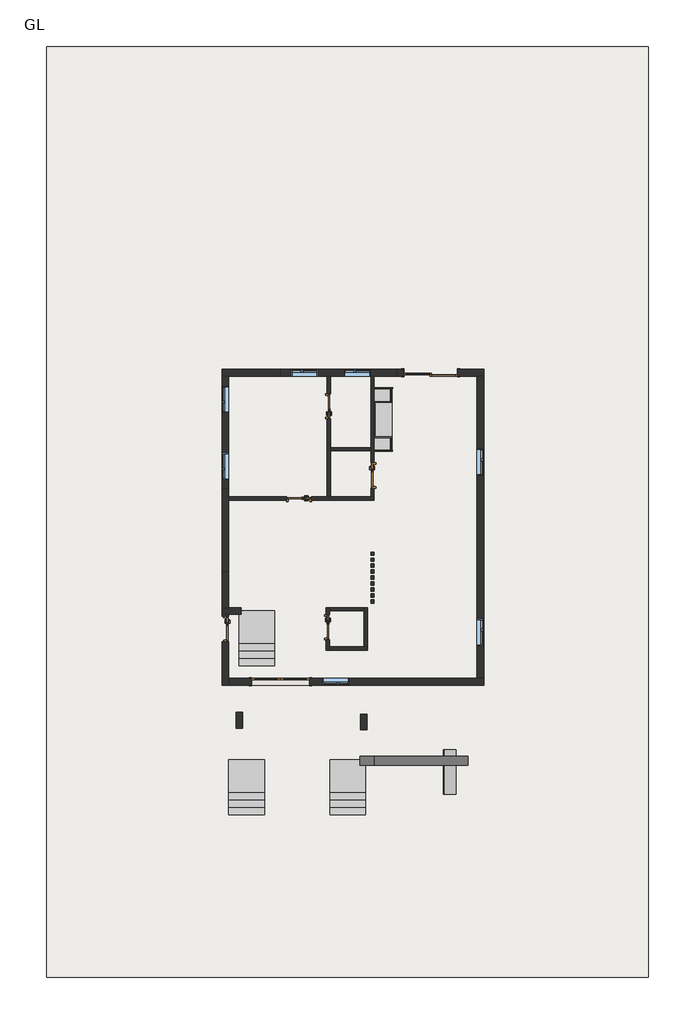
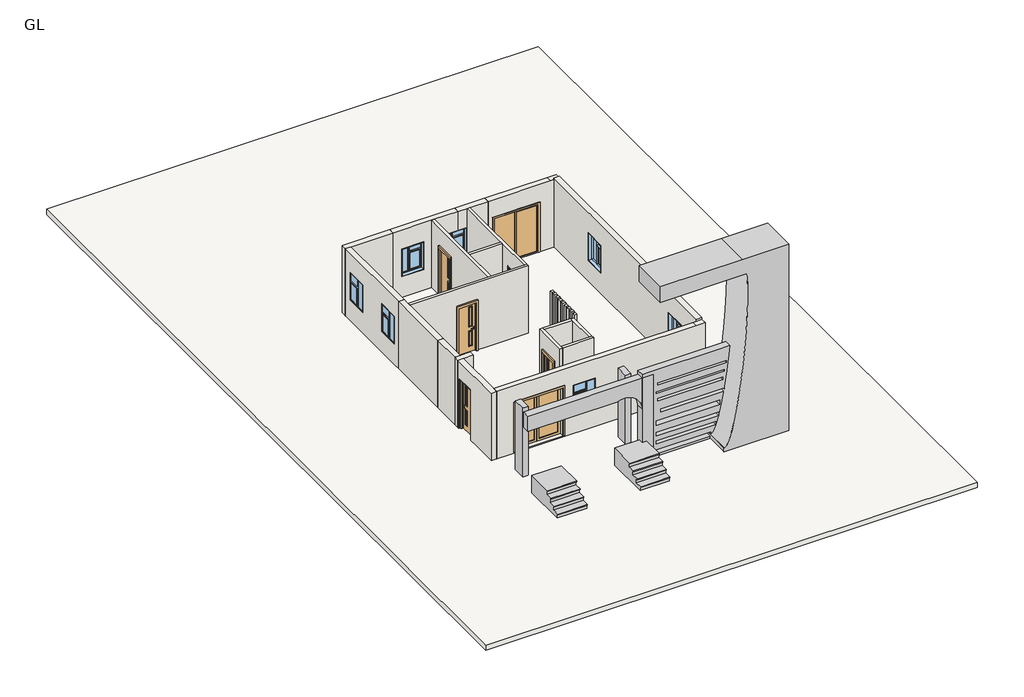
# One storey, incomplete: 28 walls, 7 doors, 7 windows, 3 geographic elements, 3 proxies, 2 columns, 2 slabs, 1 furniture element.
"""IFC4 building model written with IfcOpenShell, lengths in millimetres."""

from ifc_helpers import new_model, si_unit, frame, origin, origin_with_axes, place, context, project, spatial, polyline, outline, extrude, faceted_brep, transform, mapped, element, save
from components import generic_models_1_generic_models_1_1816b3d2, generic_models_7_generic_models_7_d72a22cb, generic_models_9_generic_models_9_71cd0b1b, door_f6d125f6, door_d4d75d1e, door_bcd1f9a3, door_10c07981, door_6f870c18, entertainment_center_with_lcd_television_8373_4fd72ac7, geographic_element_a8b2e6db, window_casement_double_sidelight_3_x_4_30e8e43c

model = new_model("IFC4")

# Units and contexts
model_context = context("Model", 3, world=origin())
ifc_project = project(units=[si_unit("LENGTHUNIT", "METRE", prefix="MILLI")], contexts=[model_context])

# Site, building, storey
site = spatial("IfcSite", under=ifc_project)
building = spatial("IfcBuilding", under=site)
storey = spatial("IfcBuildingStorey", under=building, Name="GL", Elevation=0.0)

# Proxies
placement = place(None, origin())
generic_models_1_generic_models_1_shape = generic_models_1_generic_models_1_1816b3d2(model_context)
element("IfcBuildingElementProxy", 1, Name="Generic Models 1 : Generic Models 1", ObjectType="Generic Models 1 : Generic Models 1", at=placement, inside=storey, context=model_context, shape_type="MappedRepresentation", body=[
    mapped(generic_models_1_generic_models_1_shape, transform((0.0, 0.0, 0.0), x_axis=(1.0, 0.0, 0.0), y_axis=(0.0, 1.0, 0.0), z_axis=(0.0, 0.0, 1.0))),
])
generic_models_7_generic_models_7_shape = generic_models_7_generic_models_7_d72a22cb(model_context)
element("IfcBuildingElementProxy", 2, Name="Generic Models 7 : Generic Models 7", ObjectType="Generic Models 7 : Generic Models 7", at=placement, inside=storey, context=model_context, shape_type="MappedRepresentation", body=[
    mapped(generic_models_7_generic_models_7_shape, transform((0.0, 0.0, 0.0), x_axis=(1.0, 0.0, 0.0), y_axis=(0.0, 1.0, 0.0), z_axis=(0.0, 0.0, 1.0))),
])
generic_models_9_generic_models_9_shape = generic_models_9_generic_models_9_71cd0b1b(model_context)
element("IfcBuildingElementProxy", 3, Name="Generic Models 9 : Generic Models 9", ObjectType="Generic Models 9 : Generic Models 9", at=placement, inside=storey, context=model_context, shape_type="MappedRepresentation", body=[
    mapped(generic_models_9_generic_models_9_shape, transform((0.0, -2971.8, 0.0), x_axis=(1.0, 0.0, 0.0), y_axis=(0.0, 1.0, 0.0), z_axis=(0.0, 0.0, 1.0))),
])

# Columns
element("IfcColumn", 4, ObjectType="Rectangular Column : 24\" x 24\"", at=placement, inside=storey, context=model_context, shape_type="SweptSolid", body=[
    extrude(outline(polyline([(-19619.3356484, -3061.2088252), (-19619.3356484, -3594.6088252), (-19847.9356484, -3594.6088252), (-19847.9356484, -3061.2088252), (-19619.3356484, -3061.2088252)])), origin_with_axes(), (0.0, 0.0, 1.0), 3048.0),
])
element("IfcColumn", 5, ObjectType="Rectangular Column : 24\" x 24\"", at=placement, inside=storey, context=model_context, shape_type="SweptSolid", body=[
    extrude(outline(polyline([(-15377.5356484, -3124.7088252), (-15377.5356484, -3658.1088252), (-15606.1356484, -3658.1088252), (-15606.1356484, -3124.7088252), (-15377.5356484, -3124.7088252)])), origin_with_axes(), (0.0, 0.0, 1.0), 3048.0),
])

# Doors
door_shape = door_f6d125f6(model_context)
element("IfcDoor", 6, ObjectType="Door-Double-Glass : 6'6\" x7'", at=placement, inside=storey, context=model_context, shape_type="MappedRepresentation", body=[
    mapped(door_shape, transform((-18323.9356484, -2015.8400751, 50.8), x_axis=(1.0, 0.0, 0.0), y_axis=(0.0, 1.0, 0.0), z_axis=(0.0, 0.0, 1.0))),
])
door_2_shape = door_d4d75d1e(model_context)
element("IfcDoor", 7, ObjectType="Door-Double-Sliding : 72\" x 84\"", at=placement, inside=storey, context=model_context, shape_type="MappedRepresentation", body=[
    mapped(door_2_shape, transform((-13205.8356484, 8635.4911249, 0.0), x_axis=(-1.0, 0.0, 0.0), y_axis=(0.0, -1.0, 0.0), z_axis=(0.0, 0.0, 1.0))),
])
door_3_shape = door_bcd1f9a3(model_context)
element("IfcDoor", 8, ObjectType="Door-Passage-Single-Two_Lite_Narrow : 2'6\"x 7' 2", at=placement, inside=storey, context=model_context, shape_type="MappedRepresentation", body=[
    mapped(door_3_shape, transform((-15187.0356484, 5009.6411748, 0.0), x_axis=(0.0, -1.0, 0.0), y_axis=(1.0, 0.0, 0.0), z_axis=(0.0, 0.0, 1.0))),
])
element("IfcDoor", 9, ObjectType="Door-Passage-Single-Two_Lite_Narrow : 2'6\"x 7' 2", at=placement, inside=storey, context=model_context, shape_type="MappedRepresentation", body=[
    mapped(door_3_shape, transform((-17695.2856484, 4215.8911748, 0.0), x_axis=(-1.0, 0.0, 0.0), y_axis=(0.0, -1.0, 0.0), z_axis=(0.0, 0.0, 1.0))),
])
element("IfcDoor", 10, ObjectType="Door-Passage-Single-Two_Lite_Narrow : 2'6\"x 7' 2", at=placement, inside=storey, context=model_context, shape_type="MappedRepresentation", body=[
    mapped(door_3_shape, transform((-16685.6356484, 7365.4911249, 0.0), x_axis=(0.0, 1.0, 0.0), y_axis=(-1.0, 0.0, 0.0), z_axis=(0.0, 0.0, 1.0))),
])
door_4_shape = door_10c07981(model_context)
element("IfcDoor", 11, ObjectType="Door-Passage-Single-Two_Lite_Narrow : 2'6\"x 7' 2", at=placement, inside=storey, context=model_context, shape_type="MappedRepresentation", body=[
    mapped(door_4_shape, transform((-16723.7356484, -159.2588252, 0.0), x_axis=(0.0, -1.0, 0.0), y_axis=(1.0, 0.0, 0.0), z_axis=(0.0, 0.0, 1.0))),
])
door_5_shape = door_6f870c18(model_context)
element("IfcDoor", 12, ObjectType="Door-Passage-Single-Two_Lite_Narrow : 2'6\"x 7' 2", at=placement, inside=storey, context=model_context, shape_type="MappedRepresentation", body=[
    mapped(door_5_shape, transform((-20209.8856484, -216.4088252, 0.0), x_axis=(0.0, -1.0, 0.0), y_axis=(1.0, 0.0, 0.0), z_axis=(0.0, 0.0, 1.0))),
])

# Furniture
entertainment_center_with_lcd_television_8373_shape = entertainment_center_with_lcd_television_8373_4fd72ac7(model_context)
element("IfcFurniture", 13, ObjectType="ENTERTAINMENT_CENTER_WITH_LCD_TELEVISION_8373", at=placement, inside=storey, context=model_context, shape_type="MappedRepresentation", body=[
    mapped(entertainment_center_with_lcd_television_8373_shape, transform((-15136.2356484, 6908.2911748, 0.0), x_axis=(0.0, 1.0, 0.0), y_axis=(-1.0, 0.0, 0.0), z_axis=(0.0, 0.0, 1.0))),
])

# Geographic elements
geographic_element_shape = geographic_element_a8b2e6db(model_context)
element("IfcGeographicElement", 14, ObjectType="Precast Steps : 3\"", at=placement, inside=storey, context=model_context, shape_type="MappedRepresentation", body=[
    mapped(geographic_element_shape, transform((-19101.0414528, 393.1911748, 50.8), x_axis=(1.0, 0.0, 0.0), y_axis=(0.0, 1.0, 0.0), z_axis=(0.0, 0.0, 1.0))),
])
element("IfcGeographicElement", 15, ObjectType="Precast Steps : 3\"", at=placement, inside=storey, context=model_context, shape_type="MappedRepresentation", body=[
    mapped(geographic_element_shape, transform((-16002.2414528, -4674.1088252, 50.8), x_axis=(1.0, 0.0, 0.0), y_axis=(0.0, 1.0, 0.0), z_axis=(0.0, 0.0, 1.0))),
])
element("IfcGeographicElement", 16, ObjectType="Precast Steps : 3\"", at=placement, inside=storey, context=model_context, shape_type="MappedRepresentation", body=[
    mapped(geographic_element_shape, transform((-19450.2914528, -4674.1088252, 50.8), x_axis=(1.0, 0.0, 0.0), y_axis=(0.0, 1.0, 0.0), z_axis=(0.0, 0.0, 1.0))),
])

# Slabs
element("IfcSlab", 17, ObjectType="LW Concrete on Metal Deck", at=placement, inside=storey, context=model_context, shape_type="SweptSolid", body=[
    extrude(outline(polyline([(-5798.8898438, 19613.5180321), (-5798.8898438, -12085.6819679), (-26299.5358231, -12085.6819679), (-26299.5358231, 19613.5180321), (-5798.8898438, 19613.5180321)])), frame((0.0, 0.0, -228.6), z_axis=(0.0, 0.0, 1.0), x_axis=(1.0, 0.0, 0.0)), (0.0, 0.0, 1.0), 228.6),
])
element("IfcSlab", 18, ObjectType="LW Concrete on Metal Deck", at=placement, inside=storey, context=model_context, shape_type="SweptSolid", body=[
    extrude(outline(polyline([(-15009.2356484, 8622.7911748), (-15009.2356484, 659.8911748), (-20317.8358231, 659.8911748), (-20317.8358231, 8622.7911748), (-15009.2356484, 8622.7911748)])), frame((0.0, 0.0, -228.6), z_axis=(0.0, 0.0, 1.0), x_axis=(1.0, 0.0, 0.0)), (0.0, 0.0, 1.0), 228.6),
])

# Walls
element("IfcWall", 19, ObjectType="Generic - 4.5\"", at=placement, inside=storey, context=model_context, shape_type="Brep", body=[
    faceted_brep([(-16736.4356484, 8394.1911249, 2971.8), (-16736.4356484, 8394.1911249, 0.0), (-16736.4356484, 7797.2911249, 0.0), (-16736.4356484, 7797.2911249, 2235.2), (-16736.4356484, 6933.6911249, 2235.2), (-16736.4356484, 6933.6911249, 0.0), (-16736.4356484, 4279.3911748, 0.0), (-16736.4356484, 4279.3911748, 2971.8), (-16622.1356484, 8394.1911249, 0.0), (-16622.1356484, 8394.1911249, 2971.8), (-16622.1356484, 5955.7911748, 2971.8), (-16622.1356484, 5841.4911748, 2971.8), (-16622.1356484, 4279.3911748, 2971.8), (-16622.1356484, 4279.3911748, 0.0), (-16622.1356484, 5841.4911748, 0.0), (-16622.1356484, 5955.7911748, 0.0), (-16622.1356484, 6933.6911249, 0.0), (-16622.1356484, 6933.6911249, 2235.2), (-16622.1356484, 7797.2911249, 2235.2), (-16622.1356484, 7797.2911249, 0.0)], [[[0, 1, 2, 3, 4, 5, 6, 7]], [[8, 9, 10, 11, 12, 13, 14, 15, 16, 17, 18, 19]], [[1, 8, 19, 2]], [[13, 6, 5, 16, 15, 14]], [[1, 0, 9, 8]], [[7, 6, 13, 12]], [[18, 3, 2, 19]], [[3, 18, 17, 4]], [[4, 17, 16, 5]], [[0, 7, 12, 11, 10, 9]]]),
])
element("IfcWall", 20, ObjectType="Generic - 4.5\"", at=placement, inside=storey, context=model_context, shape_type="Brep", body=[
    faceted_brep([(-20089.2356521, 4165.0911748, 2971.8), (-20089.2356521, 4165.0911748, 0.0), (-18127.0856484, 4165.0911748, 0.0), (-18127.0856484, 4165.0911748, 2235.2), (-17263.4856484, 4165.0911748, 2235.2), (-17263.4856484, 4165.0911748, 0.0), (-15136.2356484, 4165.0911748, 0.0), (-15136.2356484, 4165.0911748, 2971.8), (-20089.2356521, 4279.3911748, 0.0), (-20089.2356521, 4279.3911748, 2971.8), (-16736.4356484, 4279.3911748, 2971.8), (-16622.1356484, 4279.3911748, 2971.8), (-15250.5356484, 4279.3911748, 2971.8), (-15136.2356484, 4279.3911748, 2971.8), (-15136.2356484, 4279.3911748, 0.0), (-15250.5356484, 4279.3911748, 0.0), (-16622.1356484, 4279.3911748, 0.0), (-16736.4356484, 4279.3911748, 0.0), (-17263.4856484, 4279.3911748, 0.0), (-17263.4856484, 4279.3911748, 2235.2), (-18127.0856484, 4279.3911748, 2235.2), (-18127.0856484, 4279.3911748, 0.0)], [[[0, 1, 2, 3, 4, 5, 6, 7]], [[8, 9, 10, 11, 12, 13, 14, 15, 16, 17, 18, 19, 20, 21]], [[1, 8, 21, 2]], [[14, 6, 5, 18, 17, 16, 15]], [[1, 0, 9, 8]], [[7, 6, 14, 13]], [[20, 3, 2, 21]], [[3, 20, 19, 4]], [[4, 19, 18, 5]], [[0, 7, 13, 12, 11, 10, 9]]]),
])
element("IfcWall", 21, ObjectType="Generic - 4.5\"", at=placement, inside=storey, context=model_context, shape_type="Brep", body=[
    faceted_brep([(-15136.2356484, 4279.3911748, 2971.8), (-15136.2356484, 4279.3911748, 0.0), (-15136.2356484, 4577.8411748, 0.0), (-15136.2356484, 4577.8411748, 2235.2), (-15136.2356484, 5441.4411748, 2235.2), (-15136.2356484, 5441.4411748, 0.0), (-15136.2356484, 8394.1911249, 0.0), (-15136.2356484, 8394.1911249, 2971.8), (-15250.5356484, 4279.3911748, 0.0), (-15250.5356484, 4279.3911748, 2971.8), (-15250.5356484, 5841.4911748, 2971.8), (-15250.5356484, 5955.7911748, 2971.8), (-15250.5356484, 8394.1911249, 2971.8), (-15250.5356484, 8394.1911249, 0.0), (-15250.5356484, 5955.7911748, 0.0), (-15250.5356484, 5841.4911748, 0.0), (-15250.5356484, 5441.4411748, 0.0), (-15250.5356484, 5441.4411748, 2235.2), (-15250.5356484, 4577.8411748, 2235.2), (-15250.5356484, 4577.8411748, 0.0)], [[[0, 1, 2, 3, 4, 5, 6, 7]], [[8, 9, 10, 11, 12, 13, 14, 15, 16, 17, 18, 19]], [[1, 8, 19, 2]], [[13, 6, 5, 16, 15, 14]], [[1, 0, 9, 8]], [[7, 6, 13, 12]], [[18, 3, 2, 19]], [[3, 18, 17, 4]], [[4, 17, 16, 5]], [[0, 7, 12, 11, 10, 9]]]),
])
element("IfcWall", 22, ObjectType="Generic - 4.5\"", at=placement, inside=storey, context=model_context, shape_type="SweptSolid", body=[
    extrude(outline(polyline([(-15250.5356484, 5841.4911748), (-16622.1356484, 5841.4911748), (-16622.1356484, 5955.7911748), (-15250.5356484, 5955.7911748), (-15250.5356484, 5841.4911748)])), origin_with_axes(), (0.0, 0.0, 1.0), 2971.8),
])
element("IfcWall", 23, ObjectType="Generic - 4.5\"", at=placement, inside=storey, context=model_context, shape_type="SweptSolid", body=[
    extrude(outline(polyline([(-15136.2356484, 2285.4911748), (-15250.5356484, 2285.4911748), (-15250.5356484, 2399.7911748), (-15136.2356484, 2399.7911748), (-15136.2356484, 2285.4911748)])), origin_with_axes(), (0.0, 0.0, 1.0), 2971.8),
])
element("IfcWall", 24, ObjectType="Generic - 4.5\"", at=placement, inside=storey, context=model_context, shape_type="SweptSolid", body=[
    extrude(outline(polyline([(-15136.2356484, 2082.2911748), (-15250.5356484, 2082.2911748), (-15250.5356484, 2196.5911748), (-15136.2356484, 2196.5911748), (-15136.2356484, 2082.2911748)])), origin_with_axes(), (0.0, 0.0, 1.0), 2971.8),
])
element("IfcWall", 25, ObjectType="Generic - 4.5\"", at=placement, inside=storey, context=model_context, shape_type="SweptSolid", body=[
    extrude(outline(polyline([(-15136.2356484, 1879.0911748), (-15250.5356484, 1879.0911748), (-15250.5356484, 1993.3911748), (-15136.2356484, 1993.3911748), (-15136.2356484, 1879.0911748)])), origin_with_axes(), (0.0, 0.0, 1.0), 2971.8),
])
element("IfcWall", 26, ObjectType="Generic - 4.5\"", at=placement, inside=storey, context=model_context, shape_type="SweptSolid", body=[
    extrude(outline(polyline([(-15136.2356484, 1675.8911748), (-15250.5356484, 1675.8911748), (-15250.5356484, 1790.1911748), (-15136.2356484, 1790.1911748), (-15136.2356484, 1675.8911748)])), origin_with_axes(), (0.0, 0.0, 1.0), 2971.8),
])
element("IfcWall", 27, ObjectType="Generic - 4.5\"", at=placement, inside=storey, context=model_context, shape_type="SweptSolid", body=[
    extrude(outline(polyline([(-15136.2356484, 1472.6911748), (-15250.5356484, 1472.6911748), (-15250.5356484, 1586.9911748), (-15136.2356484, 1586.9911748), (-15136.2356484, 1472.6911748)])), origin_with_axes(), (0.0, 0.0, 1.0), 2971.8),
])
element("IfcWall", 28, ObjectType="Generic - 4.5\"", at=placement, inside=storey, context=model_context, shape_type="SweptSolid", body=[
    extrude(outline(polyline([(-15136.2356484, 1269.4911748), (-15250.5356484, 1269.4911748), (-15250.5356484, 1383.7911748), (-15136.2356484, 1383.7911748), (-15136.2356484, 1269.4911748)])), origin_with_axes(), (0.0, 0.0, 1.0), 2971.8),
])
element("IfcWall", 29, ObjectType="Generic - 4.5\"", at=placement, inside=storey, context=model_context, shape_type="SweptSolid", body=[
    extrude(outline(polyline([(-15136.2356484, 1066.2911748), (-15250.5356484, 1066.2911748), (-15250.5356484, 1180.5911748), (-15136.2356484, 1180.5911748), (-15136.2356484, 1066.2911748)])), origin_with_axes(), (0.0, 0.0, 1.0), 2971.8),
])
element("IfcWall", 30, ObjectType="Generic - 4.5\"", at=placement, inside=storey, context=model_context, shape_type="SweptSolid", body=[
    extrude(outline(polyline([(-15136.2356484, 863.0911748), (-15250.5356484, 863.0911748), (-15250.5356484, 977.3911748), (-15136.2356484, 977.3911748), (-15136.2356484, 863.0911748)])), origin_with_axes(), (0.0, 0.0, 1.0), 2971.8),
])
element("IfcWall", 31, ObjectType="Generic - 4.5\"", at=placement, inside=storey, context=model_context, shape_type="SweptSolid", body=[
    extrude(outline(polyline([(-15136.2356484, 659.8911748), (-15250.5356484, 659.8911748), (-15250.5356484, 774.1911748), (-15136.2356484, 774.1911748), (-15136.2356484, 659.8911748)])), origin_with_axes(), (0.0, 0.0, 1.0), 2971.8),
])
element("IfcWall", 32, ObjectType="Generic - 4.5\"", at=placement, inside=storey, context=model_context, shape_type="Brep", body=[
    faceted_brep([(-16774.5356484, -940.3088251, 0.0), (-16774.5356484, -940.3088251, 2971.8), (-16774.5356484, 507.4911748, 2971.8), (-16774.5356484, 507.4911748, 0.0), (-16774.5356484, 272.5411748, 0.0), (-16774.5356484, 272.5411748, 2235.2), (-16774.5356484, -591.0588252, 2235.2), (-16774.5356484, -591.0588252, 0.0), (-16660.2356484, -940.3088251, 2971.8), (-16660.2356484, -940.3088251, 0.0), (-16660.2356484, -826.0088251, 0.0), (-16660.2356484, -591.0588252, 0.0), (-16660.2356484, -591.0588252, 2235.2), (-16660.2356484, 272.5411748, 2235.2), (-16660.2356484, 272.5411748, 0.0), (-16660.2356484, 393.1911748, 0.0), (-16660.2356484, 507.4911748, 0.0), (-16660.2356484, 507.4911748, 2971.8), (-16660.2356484, 393.1911748, 2971.8), (-16660.2356484, -826.0088251, 2971.8)], [[[0, 1, 2, 3, 4, 5, 6, 7]], [[8, 9, 10, 11, 12, 13, 14, 15, 16, 17, 18, 19]], [[9, 0, 7, 11, 10]], [[3, 16, 15, 14, 4]], [[1, 0, 9, 8]], [[3, 2, 17, 16]], [[6, 12, 11, 7]], [[12, 6, 5, 13]], [[13, 5, 4, 14]], [[2, 1, 8, 19, 18, 17]]]),
])
element("IfcWall", 33, ObjectType="Generic - 4.5\"", at=placement, inside=storey, context=model_context, shape_type="Brep", body=[
    faceted_brep([(-16660.2356484, -940.3088251, 0.0), (-15364.8356484, -940.3088251, 0.0), (-15364.8356484, -940.3088251, 2971.8), (-16660.2356484, -940.3088251, 2971.8), (-16660.2356484, -826.0088251, 0.0), (-16660.2356484, -826.0088251, 2971.8), (-15479.1356484, -826.0088251, 2971.8), (-15364.8356484, -826.0088251, 2971.8), (-15364.8356484, -826.0088251, 0.0), (-15479.1356484, -826.0088251, 0.0)], [[[0, 1, 2, 3]], [[4, 5, 6, 7, 8, 9]], [[1, 0, 4, 9, 8]], [[0, 3, 5, 4]], [[2, 1, 8, 7]], [[3, 2, 7, 6, 5]]]),
])
element("IfcWall", 34, ObjectType="Generic - 4.5\"", at=placement, inside=storey, context=model_context, shape_type="Brep", body=[
    faceted_brep([(-15364.8356484, -826.0088251, 0.0), (-15364.8356484, 507.4911748, 0.0), (-15364.8356484, 507.4911748, 2971.8), (-15364.8356484, -826.0088251, 2971.8), (-15479.1356484, -826.0088251, 0.0), (-15479.1356484, -826.0088251, 2971.8), (-15479.1356484, 393.1911748, 2971.8), (-15479.1356484, 507.4911748, 2971.8), (-15479.1356484, 507.4911748, 0.0), (-15479.1356484, 393.1911748, 0.0)], [[[0, 1, 2, 3]], [[4, 5, 6, 7, 8, 9]], [[1, 0, 4, 9, 8]], [[0, 3, 5, 4]], [[2, 1, 8, 7]], [[3, 2, 7, 6, 5]]]),
])
element("IfcWall", 35, ObjectType="Generic - 4.5\"", at=placement, inside=storey, context=model_context, shape_type="SweptSolid", body=[
    extrude(outline(polyline([(-16660.2356484, 507.4911748), (-15479.1356484, 507.4911748), (-15479.1356484, 393.1911748), (-16660.2356484, 393.1911748), (-16660.2356484, 507.4911748)])), origin_with_axes(), (0.0, 0.0, 1.0), 2971.8),
])
element("IfcWall", 36, ObjectType="Generic - 9\"Masonry 2", at=placement, inside=storey, context=model_context, shape_type="Brep", body=[
    faceted_brep([(-20317.8358231, 8394.1911748, 0.0), (-20089.2358231, 8394.1911748, 0.0), (-18336.6356484, 8394.1911748, 0.0), (-18336.6356484, 8394.1911748, 2971.8), (-20089.2358231, 8394.1911748, 2971.8), (-20317.8358231, 8394.1911748, 2971.8), (-20317.8358231, 8622.7911748, 0.0), (-20317.8358231, 8622.7911748, 2971.8), (-18336.6356484, 8622.7911748, 2971.8), (-18336.6356484, 8622.7911748, 0.0)], [[[0, 1, 2, 3, 4, 5]], [[6, 7, 8, 9]], [[2, 1, 0, 6, 9]], [[3, 2, 9, 8]], [[0, 5, 7, 6]], [[5, 4, 3, 8, 7]]]),
])
element("IfcWall", 37, ObjectType="Generic - 9\"Masonry 2", at=placement, inside=storey, context=model_context, shape_type="Brep", body=[
    faceted_brep([(-18336.6356484, 8394.1911249, 0.0), (-16736.4356484, 8394.1911249, 0.0), (-16622.1356484, 8394.1911249, 0.0), (-15630.0916974, 8394.1911249, 0.0), (-15630.0916974, 8394.1911249, 914.4), (-16163.4916974, 8394.1911249, 914.4), (-16163.4916974, 8394.1911249, 2133.6), (-15630.0916974, 8394.1911249, 2133.6), (-15630.0916974, 8394.1911249, 2971.8), (-16622.1356484, 8394.1911249, 2971.8), (-16736.4356484, 8394.1911249, 2971.8), (-18336.6356484, 8394.1911249, 2971.8), (-17050.7606484, 8394.1911249, 2133.6), (-17050.7606484, 8394.1911249, 914.4), (-17965.1606484, 8394.1911249, 914.4), (-17965.1606484, 8394.1911249, 2133.6), (-15630.0916974, 8622.7911249, 0.0), (-18336.6356484, 8622.7911249, 0.0), (-18336.6356484, 8622.7911249, 2971.8), (-15630.0916974, 8622.7911249, 2971.8), (-15630.0916974, 8622.7911249, 2133.6), (-16163.4916974, 8622.7911249, 2133.6), (-16163.4916974, 8622.7911249, 914.4), (-15630.0916974, 8622.7911249, 914.4), (-17050.7606484, 8622.7911249, 2133.6), (-17965.1606484, 8622.7911249, 2133.6), (-17965.1606484, 8622.7911249, 914.4), (-17050.7606484, 8622.7911249, 914.4)], [[[0, 1, 2, 3, 4, 5, 6, 7, 8, 9, 10, 11], [12, 13, 14, 15]], [[16, 17, 18, 19, 20, 21, 22, 23], [24, 25, 26, 27]], [[3, 2, 1, 0, 17, 16]], [[3, 16, 23, 4]], [[19, 8, 7, 20]], [[0, 11, 18, 17]], [[13, 12, 24, 27]], [[14, 13, 27, 26]], [[15, 14, 26, 25]], [[12, 15, 25, 24]], [[22, 5, 4, 23]], [[5, 22, 21, 6]], [[6, 21, 20, 7]], [[11, 10, 9, 8, 19, 18]]]),
])
element("IfcWall", 38, ObjectType="Generic - 9\"Masonry 2", at=placement, inside=storey, context=model_context, shape_type="Brep", body=[
    faceted_brep([(-15630.0916974, 8394.1911249, 0.0), (-15250.5356484, 8394.1911249, 0.0), (-15136.2356484, 8394.1911249, 0.0), (-14374.2356484, 8394.1911249, 0.0), (-14374.2356484, 8394.1911249, 2971.8), (-15136.2356484, 8394.1911249, 2971.8), (-15250.5356484, 8394.1911249, 2971.8), (-15630.0916974, 8394.1911249, 2971.8), (-15630.0916974, 8394.1911249, 2133.6), (-15249.0916974, 8394.1911249, 2133.6), (-15249.0916974, 8394.1911249, 914.4), (-15630.0916974, 8394.1911249, 914.4), (-14374.2356484, 8622.7911249, 0.0), (-15630.0916974, 8622.7911249, 0.0), (-15630.0916974, 8622.7911249, 914.4), (-15249.0916974, 8622.7911249, 914.4), (-15249.0916974, 8622.7911249, 2133.6), (-15630.0916974, 8622.7911249, 2133.6), (-15630.0916974, 8622.7911249, 2971.8), (-14374.2356484, 8622.7911249, 2971.8)], [[[0, 1, 2, 3, 4, 5, 6, 7, 8, 9, 10, 11]], [[12, 13, 14, 15, 16, 17, 18, 19]], [[3, 2, 1, 0, 13, 12]], [[4, 3, 12, 19]], [[13, 0, 11, 14]], [[7, 18, 17, 8]], [[9, 16, 15, 10]], [[10, 15, 14, 11]], [[16, 9, 8, 17]], [[7, 6, 5, 4, 19, 18]]]),
])
element("IfcWall", 39, ObjectType="Generic - 9\"Masonry 2", at=placement, inside=storey, context=model_context, shape_type="Brep", body=[
    faceted_brep([(-14374.2356484, 8394.1911249, 0.0), (-14120.2356484, 8394.1911249, 0.0), (-14120.2356484, 8394.1911249, 2133.6), (-12291.4356484, 8394.1911249, 2133.6), (-12291.4356484, 8394.1911249, 0.0), (-11631.0356484, 8394.1911249, 0.0), (-11402.4356484, 8394.1911249, 0.0), (-11402.4356484, 8394.1911249, 2971.8), (-11770.7356484, 8394.1911249, 2971.8), (-14374.2356484, 8394.1911249, 2971.8), (-14120.2356484, 8622.7911249, 2133.6), (-14120.2356484, 8622.7911249, 0.0), (-14374.2356484, 8622.7911249, 0.0), (-14374.2356484, 8622.7911249, 2971.8), (-11770.7356484, 8622.7911249, 2971.8), (-11402.4356484, 8622.7911249, 2971.8), (-11402.4356484, 8622.7911249, 0.0), (-12291.4356484, 8622.7911249, 0.0), (-12291.4356484, 8622.7911249, 2133.6)], [[[0, 1, 2, 3, 4, 5, 6, 7, 8, 9]], [[10, 11, 12, 13, 14, 15, 16, 17, 18]], [[17, 16, 6, 5, 4]], [[12, 11, 1, 0]], [[0, 9, 13, 12]], [[7, 6, 16, 15]], [[4, 3, 18, 17]], [[2, 1, 11, 10]], [[3, 2, 10, 18]], [[8, 7, 15, 14]], [[9, 8, 14, 13]]]),
])
element("IfcWall", 40, ObjectType="Generic - 9\"Masonry 2", at=placement, inside=storey, context=model_context, shape_type="Brep", body=[
    faceted_brep([(-11631.0356484, 8394.1911249, 0.0), (-11631.0356484, -1899.1588251, 0.0), (-11631.0356484, -1899.1588251, 3048.0), (-11631.0356484, 8394.1911249, 3048.0), (-11631.0356484, -794.2588251, 2133.6), (-11631.0356484, -794.2588251, 914.4), (-11631.0356484, 120.1411749, 914.4), (-11631.0356484, 120.1411749, 2133.6), (-11631.0356484, 5003.2911249, 2133.6), (-11631.0356484, 5003.2911249, 914.4), (-11631.0356484, 5917.6911249, 914.4), (-11631.0356484, 5917.6911249, 2133.6), (-11402.4356484, -1899.1588251, 0.0), (-11402.4356484, 8394.1911249, 0.0), (-11402.4356484, 8394.1911249, 2971.8), (-11402.4356484, 8394.1911249, 3048.0), (-11402.4356484, -1899.1588251, 3048.0), (-11402.4356484, -1899.1588251, 2971.8), (-11402.4356484, -794.2588251, 914.4), (-11402.4356484, -794.2588251, 2133.6), (-11402.4356484, 120.1411749, 2133.6), (-11402.4356484, 120.1411749, 914.4), (-11402.4356484, 5003.2911249, 914.4), (-11402.4356484, 5003.2911249, 2133.6), (-11402.4356484, 5917.6911249, 2133.6), (-11402.4356484, 5917.6911249, 914.4)], [[[0, 1, 2, 3], [4, 5, 6, 7], [8, 9, 10, 11]], [[12, 13, 14, 15, 16, 17], [18, 19, 20, 21], [22, 23, 24, 25]], [[1, 0, 13, 12]], [[3, 2, 16, 15]], [[0, 3, 15, 14, 13]], [[2, 1, 12, 17, 16]], [[4, 19, 18, 5]], [[5, 18, 21, 6]], [[6, 21, 20, 7]], [[19, 4, 7, 20]], [[8, 23, 22, 9]], [[9, 22, 25, 10]], [[10, 25, 24, 11]], [[23, 8, 11, 24]]]),
])
element("IfcWall", 41, ObjectType="Generic - 9\"Masonry 2", at=placement, inside=storey, context=model_context, shape_type="Brep", body=[
    faceted_brep([(-19670.1356484, 507.4911748, 0.0), (-20089.2356484, 507.4911748, 0.0), (-20317.8356484, 507.4911748, 0.0), (-20317.8356484, 507.4911748, 2971.8), (-20089.2356484, 507.4911748, 2971.8), (-19670.1356484, 507.4911748, 2971.8), (-19670.1356484, 278.8911748, 0.0), (-19670.1356484, 278.8911748, 2971.8), (-20089.2356484, 278.8911748, 2971.8), (-20317.8356484, 278.8911748, 2971.8), (-20317.8356484, 278.8911748, 0.0), (-20089.2356484, 278.8911748, 0.0)], [[[0, 1, 2, 3, 4, 5]], [[6, 7, 8, 9, 10, 11]], [[2, 1, 0, 6, 11, 10]], [[0, 5, 7, 6]], [[3, 2, 10, 9]], [[5, 4, 3, 9, 8, 7]]]),
])
element("IfcWall", 42, ObjectType="Generic - 9\"Masonry 2", at=placement, inside=storey, context=model_context, shape_type="SweptSolid", body=[
    extrude(outline(polyline([(-20089.2356484, 1726.6911748), (-20089.2356484, 507.4911748), (-20317.8356484, 507.4911748), (-20317.8356484, 1726.6911748), (-20089.2356484, 1726.6911748)])), origin_with_axes(), (0.0, 0.0, 1.0), 2971.8),
])
element("IfcWall", 43, ObjectType="Generic - 9\"Masonry 2", at=placement, inside=storey, context=model_context, shape_type="Brep", body=[
    faceted_brep([(-20089.2356521, 1726.6911748, 0.0), (-20089.2356521, 4165.0911748, 0.0), (-20089.2356521, 4279.3911748, 0.0), (-20089.2356521, 4554.7078432, 0.0), (-20089.2356521, 4554.7078432, 2971.8), (-20089.2356521, 4279.3911748, 2971.8), (-20089.2356521, 4165.0911748, 2971.8), (-20089.2356521, 1726.6911748, 2971.8), (-20317.8356521, 1726.6911748, 0.0), (-20317.8356521, 1726.6911748, 2971.8), (-20317.8356521, 4554.7078432, 2971.8), (-20317.8356521, 4554.7078432, 0.0)], [[[0, 1, 2, 3, 4, 5, 6, 7]], [[8, 9, 10, 11]], [[3, 2, 1, 0, 8, 11]], [[4, 3, 11, 10]], [[0, 7, 9, 8]], [[7, 6, 5, 4, 10, 9]]]),
])
element("IfcWall", 44, ObjectType="Generic - 9\"Masonry 2", at=placement, inside=storey, context=model_context, shape_type="SweptSolid", body=[
    extrude(outline(polyline([(4554.7078432, 0.0), (4554.7078432, 2971.8), (8394.1911748, 2971.8), (8394.1911748, 0.0), (4554.7078432, 0.0)]), holes=[polyline([(5773.9078432, 2133.6), (4859.5078432, 2133.6), (4859.5078432, 914.4), (5773.9078432, 914.4), (5773.9078432, 2133.6)]), polyline([(8051.2911748, 2133.6), (7136.8911748, 2133.6), (7136.8911748, 914.4), (8051.2911748, 914.4), (8051.2911748, 2133.6)])]), frame((-20317.8358231, 0.0, 0.0), z_axis=(1.0, 0.0, 0.0), x_axis=(0.0, 1.0, 0.0)), (0.0, 0.0, 1.0), 228.6),
])
element("IfcWall", 45, ObjectType="Generic - 9\"Masonry 2", at=placement, inside=storey, context=model_context, shape_type="Brep", body=[
    faceted_brep([(-20317.8356484, 278.8911748, 2971.8), (-20317.8356484, 278.8911748, 0.0), (-20317.8356484, 215.3911748, 0.0), (-20317.8356484, 215.3911748, 2235.2), (-20317.8356484, -648.2088252, 2235.2), (-20317.8356484, -648.2088252, 0.0), (-20317.8356484, -2127.7588251, 0.0), (-20317.8356484, -2127.7588251, 2971.8), (-20089.2356484, 278.8911748, 0.0), (-20089.2356484, 278.8911748, 2971.8), (-20089.2356484, -1899.1588251, 2971.8), (-20089.2356484, -2127.7588251, 2971.8), (-20089.2356484, -2127.7588251, 0.0), (-20089.2356484, -1899.1588251, 0.0), (-20089.2356484, -648.2088252, 0.0), (-20089.2356484, -648.2088252, 2235.2), (-20089.2356484, 215.3911748, 2235.2), (-20089.2356484, 215.3911748, 0.0)], [[[0, 1, 2, 3, 4, 5, 6, 7]], [[8, 9, 10, 11, 12, 13, 14, 15, 16, 17]], [[1, 8, 17, 2]], [[12, 6, 5, 14, 13]], [[1, 0, 9, 8]], [[7, 6, 12, 11]], [[4, 15, 14, 5]], [[15, 4, 3, 16]], [[16, 3, 2, 17]], [[0, 7, 11, 10, 9]]]),
])
element("IfcWall", 46, ObjectType="Generic - 9\"Masonry 2", at=placement, inside=storey, context=model_context, shape_type="Brep", body=[
    faceted_brep([(-20089.2356484, -2127.7588251, 0.0), (-11402.4356484, -2127.7588251, 0.0), (-11402.4356484, -2127.7588251, 2971.8), (-11770.7356484, -2127.7588251, 2971.8), (-20089.2356484, -2127.7588251, 2971.8), (-19314.5356484, -2127.7588251, 50.8), (-19314.5356484, -2127.7588251, 2184.4), (-17333.3356484, -2127.7588251, 2184.4), (-17333.3356484, -2127.7588251, 50.8), (-16901.5356484, -2127.7588251, 2133.6), (-15987.1356484, -2127.7588251, 2133.6), (-15987.1356484, -2127.7588251, 914.4), (-16901.5356484, -2127.7588251, 914.4), (-20089.2356484, -1899.1588251, 0.0), (-20089.2356484, -1899.1588251, 2971.8), (-11770.7356484, -1899.1588251, 2971.8), (-11402.4356484, -1899.1588251, 2971.8), (-11402.4356484, -1899.1588251, 0.0), (-11631.0356484, -1899.1588251, 0.0), (-19314.5356484, -1899.1588251, 50.8), (-17333.3356484, -1899.1588251, 50.8), (-17333.3356484, -1899.1588251, 2184.4), (-19314.5356484, -1899.1588251, 2184.4), (-16901.5356484, -1899.1588251, 2133.6), (-16901.5356484, -1899.1588251, 914.4), (-15987.1356484, -1899.1588251, 914.4), (-15987.1356484, -1899.1588251, 2133.6)], [[[0, 1, 2, 3, 4], [5, 6, 7, 8], [9, 10, 11, 12]], [[13, 14, 15, 16, 17, 18], [19, 20, 21, 22], [23, 24, 25, 26]], [[1, 0, 13, 18, 17]], [[0, 4, 14, 13]], [[20, 19, 5, 8]], [[21, 20, 8, 7]], [[22, 21, 7, 6]], [[19, 22, 6, 5]], [[2, 1, 17, 16]], [[3, 2, 16, 15]], [[4, 3, 15, 14]], [[24, 23, 9, 12]], [[25, 24, 12, 11]], [[26, 25, 11, 10]], [[23, 26, 10, 9]]]),
])

# Windows
window_casement_double_sidelight_3_x_4_shape = window_casement_double_sidelight_3_x_4_30e8e43c(model_context)
element("IfcWindow", 47, ObjectType="Window-Casement-Double-Sidelight : 3'x 4'", at=placement, inside=storey, context=model_context, shape_type="MappedRepresentation", body=[
    mapped(window_casement_double_sidelight_3_x_4_shape, transform((-17507.9606484, 8508.4911249, 0.0), x_axis=(1.0, 0.0, 0.0), y_axis=(0.0, 1.0, 0.0), z_axis=(0.0, 0.0, 1.0))),
])
element("IfcWindow", 48, ObjectType="Window-Casement-Double-Sidelight : 3'x 4'", at=placement, inside=storey, context=model_context, shape_type="MappedRepresentation", body=[
    mapped(window_casement_double_sidelight_3_x_4_shape, transform((-15706.2916974, 8508.4911249, 0.0), x_axis=(1.0, 0.0, 0.0), y_axis=(0.0, 1.0, 0.0), z_axis=(0.0, 0.0, 1.0))),
])
element("IfcWindow", 49, ObjectType="Window-Casement-Double-Sidelight : 3'x 4'", at=placement, inside=storey, context=model_context, shape_type="MappedRepresentation", body=[
    mapped(window_casement_double_sidelight_3_x_4_shape, transform((-11516.7356484, 5460.4911249, 0.0), x_axis=(0.0, -1.0, 0.0), y_axis=(1.0, 0.0, 0.0), z_axis=(0.0, 0.0, 1.0))),
])
element("IfcWindow", 50, ObjectType="Window-Casement-Double-Sidelight : 3'x 4'", at=placement, inside=storey, context=model_context, shape_type="MappedRepresentation", body=[
    mapped(window_casement_double_sidelight_3_x_4_shape, transform((-20203.5358231, 5316.7078432, 0.0), x_axis=(0.0, 1.0, 0.0), y_axis=(-1.0, 0.0, 0.0), z_axis=(0.0, 0.0, 1.0))),
])
element("IfcWindow", 51, ObjectType="Window-Casement-Double-Sidelight : 3'x 4'", at=placement, inside=storey, context=model_context, shape_type="MappedRepresentation", body=[
    mapped(window_casement_double_sidelight_3_x_4_shape, transform((-20203.5358231, 7594.0911748, 0.0), x_axis=(0.0, 1.0, 0.0), y_axis=(-1.0, 0.0, 0.0), z_axis=(0.0, 0.0, 1.0))),
])
element("IfcWindow", 52, ObjectType="Window-Casement-Double-Sidelight : 3'x 4'", at=placement, inside=storey, context=model_context, shape_type="MappedRepresentation", body=[
    mapped(window_casement_double_sidelight_3_x_4_shape, transform((-11516.7356484, -337.0588251, 0.0), x_axis=(0.0, -1.0, 0.0), y_axis=(1.0, 0.0, 0.0), z_axis=(0.0, 0.0, 1.0))),
])
element("IfcWindow", 53, ObjectType="Window-Casement-Double-Sidelight : 3'x 4'", at=placement, inside=storey, context=model_context, shape_type="MappedRepresentation", body=[
    mapped(window_casement_double_sidelight_3_x_4_shape, transform((-16444.3356484, -2013.4588251, 0.0), x_axis=(-1.0, 0.0, 0.0), y_axis=(0.0, -1.0, 0.0), z_axis=(0.0, 0.0, 1.0))),
])

save(model, "model.ifc")

# Revit data of these elements
# Type "Rectangular Column : 24\" x 24\""
#   Assembly Code = "B1010200"
#   Depth = 1' - 9"
#   Offset Base = 0' - 0"
#   Offset Top = 0' - 0"
#   Width = 0' - 9"
#   Material = none
# Type "Door-Double-Glass : 6'6\" x7'"
#   Type Mark = "29"
#   Construction Type Id = "opn-d45"
#   Assembly Code = "C1020"
#   Analytic Construction = "Wood frame, double glass door "
#   W = 3' - 3"
#   Thickness = 0' - 2"
#   Thermal Resistance (R) = 1.8150 (h·ft²·°F)/BTU
#   Swing Angle [instance default] = 90.00°
#   Heat Transfer Coefficient (U) = 0.5510 BTU/(h·ft²·°F)
#   Height = 7' - 0"
#   Bottom Rail = 0' - 4"
#   Top Rail = 0' - 4"
#   Stiles = 0' - 4"
#   Trim Projection = 0' - 1"
#   Trim Width = 0' - 3"
#   Width = 6' - 6"
#   Define Thermal Properties by = 1
#   Glazing = Glass
#   Panel Material = Wood - Birch - Solid Stained Light Low Gloss
#   Trim Material = Paint - Sienna
#   Visual Light Transmittance = 0
#   Solar Heat Gain Coefficient = 0
#   Function = (empty or 0)
#   Wall Closure = (empty or 0)
# Type "Door-Double-Sliding : 72\" x 84\""
#   Type Mark = "11"
#   Construction Type Id = "opn-d45"
#   Assembly Code = "C1020"
#   Analytic Construction = "Wood frame, double glass door "
#   Thickness = 0' - 2"
#   Thermal Resistance (R) = 1.8150 (h·ft²·°F)/BTU
#   Heat Transfer Coefficient (U) = 0.5510 BTU/(h·ft²·°F)
#   Height = 7' - 0"
#   Rail Width = 0' - 2"
#   Stiles = 0' - 2"
#   Trim Projection Ext = 0' - 1"
#   Trim Projection Int = 0' - 1"
#   Trim Width = 0' - 3"
#   Width = 6' - 0"
#   Define Thermal Properties by = 1
#   Glazing = Glass
#   Panel Material = Wood - Birch - Solid Stained Light Low Gloss
#   Trim Material = Paint - Sienna
#   Visual Light Transmittance = 0
#   Solar Heat Gain Coefficient = 0
#   Function = (empty or 0)
#   Wall Closure = (empty or 0)
# Type "Door-Passage-Single-Two_Lite_Narrow : 2'6\"x 7' 2"
#   Type Mark = "10"
#   Assembly Code = "B2030100"
#   Analytic Construction = "Wooden"
#   Thickness = 0' - 1 3/4"
#   Thermal Resistance (R) = 2.5876 (h·ft²·°F)/BTU
#   Swing Angle [instance default] = 90.00°
#   Strike Height = 3' - 4"
#   Rough Width [instance default] = 2' - 10"
#   Rough Height [instance default] = 7' - 4"
#   MFOpeningHeight [instance default] = 0' - 4"
#   MFOpeningWidth [instance default] = 0' - 4"
#   Heat Transfer Coefficient (U) = 0.3865 BTU/(h·ft²·°F)
#   Inset Calculate [instance default] = 0' - 4"
#   Masonry Inset [instance default] = 0' - 1"
#   Height = 7' - 0"
#   Width = 2' - 6"
#   Masonry Frame Depth = 0' - 5 3/4"
#   Masonry Frame [instance default] = yes
#   Function = 1
#   Dry Wall Frame [instance default] = no
#   Panel Material = Wood - Birch
#   Glazing = Glass
#   Glass Stop Material = Metal - Paint Finish - Grey
#   Frame Material = Metal - Paint Finish - Grey
#   Door Handle Material = Aluminum
#   Visual Light Transmittance = 0
#   Solar Heat Gain Coefficient = 0
#   Wall Closure = (empty or 0)
# Type "ENTERTAINMENT_CENTER_WITH_LCD_TELEVISION_8373"
#   TV PNL HEIGHT = 0' - 2"
#   TV LENGTH = 3' - 3"
#   TV LED HEIGHT = 0' - 1 3/128"
#   TV HEIGHT FROM TOP OF CASE = 0' - 3"
#   TV HEIGHT = 2' - 2"
#   TOP MLDG HEIGHT = 1' - 5"
#   SPEAKER PNL EDGE WIDTH = 0' - 0 1/4"
#   SHELVES FROM TOP OF CASE = 1' - 0"
#   MLDG WIDTH FROM GLASS = 0' - 0 3/4"
#   MLDG WIDTH = 0' - 2"
#   MLDG HEIGHT = 0' - 1 25/64"
#   LED TOP DISTANCE = 0' - 3 19/256"
#   GLASS SHELF THICKNESS = 0' - 0 1/8"
#   DOOR MLDG WIDTH = 0' - 0 1/2"
#   DOOR MLDG THICKNESS = 0' - 0 1/8"
#   Center Panel Height = 2' - 5"
#   WIDTH = 2' - 0"
#   PANEL THICKNESS = 0' - 0 3/4"
#   LENGTH = 7' - 0"
#   HEIGHT = 6' - 0"
#   GLASS THICKNESS = 0' - 0 1/8"
#   GLASS LENGTH = 1' - 5"
#   DOOR PNL WIDTH = 0' - 2"
#   CROWN MLDG WIDTH = 0' - 3 177/256"
#   CENTER WIDTH = 4' - 0"
#   CENTER SPEAKER HEIGHT = 0' - 8"
#   Back Panel Width = 0' - 0 1/8"
#   SIDE DOORS INCLUDED [instance default] = yes
#   MESH SPEAKER PNLS INCLUDED [instance default] = yes
#   CASE FINISH = WOOD DARK MAHOGANY
#   Default Elevation = 0
# Type "Precast Steps : 3\""
#   Assembly Code = "G"
#   Landing = 3' - 6"
#   Step Offset = 0' - 10"
#   Width = 4' - 0"
#   Material = Concrete - Precast Concrete
# Type "LW Concrete on Metal Deck"
#   Assembly Code = "B1010"
#   Function = 0
#   Layers, outside or top first: 0' - 4" "Concrete, Lightweight" (function 1); 0' - 5" "Metal Deck" (function 1)
# Type "Generic - 4.5\""
#   Assembly Code = "B2010"
#   Layers, outside or top first: 0' - 4 1/2" no material (function 1)
# Type "Generic - 9\"Masonry 2"
#   Assembly Code = "B2010"
#   Layers, outside or top first: 0' - 9" "Concrete Masonry Units" (function 1)
# Type "Window-Casement-Double-Sidelight : 3'x 4'"
#   Type Mark = "22"
#   Fire Rating = "0.5h"
#   Assembly Code = "B2020100"
#   Analytic Construction = "Double glazing - domestic"
#   Window Inset [instance default] = 0' - 0 5/8"
#   Wall Thickness [instance default] = 0' - 6"
#   Visual Light Transmittance = 0.81
#   Transom Height Ratio = 0.3
#   Transom Height = 1' - 2.4"
#   Thermal Resistance (R) = 1.8146 (h·ft²·°F)/BTU
#   Solar Heat Gain Coefficient = 0.76
#   Side Width = 1' - 2.4"
#   Rough Width = 3' - 0 1/2"
#   Rough Height = 4' - 0 1/2"
#   Opening Window Width = 1' - 9.6"
#   Opening Window Height = 2' - 9.6"
#   Heat Transfer Coefficient (U) = 0.5511 BTU/(h·ft²·°F)
#   Height = 4' - 0"
#   Frame Gap 3 [instance default] = 0' - 1 83/128"
#   Frame Gap 2 [instance default] = 0' - 0 5/8"
#   Frame Gap 1 = 0' - 1 51/128"
#   Default Sill Height = 3' - 0"
#   Width = 3' - 0"
#   Frame Material = Metal - Aluminum
#   Glass Panel Material = Glass
#   Wall Closure = (empty or 0)
# Element 1 (IfcBuildingElementProxy, "Generic Models 1 : Generic Models 1")
#   Phase Created = New Construction
# Element 2 (IfcBuildingElementProxy, "Generic Models 7 : Generic Models 7")
#   Phase Created = New Construction
# Element 3 (IfcBuildingElementProxy, "Generic Models 9 : Generic Models 9")
#   Phase Created = New Construction
# Elements 4, 5 (IfcColumn, "Rectangular Column : 24\" x 24\"")
#   Phase Created = New Construction
# Element 6 (IfcDoor, "Door-Double-Glass : 6'6\" x7'")
#   Swing Angle = 90.00°
#   Phase Created = New Construction
#   Materials on its faces: "Wood - Birch - Solid Stained Light Low Gloss", "Paint - Sienna", "Glass"
# Element 7 (IfcDoor, "Door-Double-Sliding : 72\" x 84\"")
#   Phase Created = New Construction
#   Materials on its faces: "Paint - Sienna", "Wood - Birch - Solid Stained Light Low Gloss", "Glass"
# Elements 8, 9, 10, 11, 12 (IfcDoor, "Door-Passage-Single-Two_Lite_Narrow : 2'6\"x 7' 2")
#   Swing Angle = 90.00°
#   Rough Width = 2' - 10"
#   Rough Height = 7' - 4"
#   Masonry Inset = 0' - 1"
#   MFOpeningWidth = 0' - 4"
#   MFOpeningHeight = 0' - 4"
#   Inset Calculate = 0' - 4"
#   Masonry Frame = yes
#   Dry Wall Frame = no
#   Phase Created = New Construction
#   Materials on its faces: "Metal - Paint Finish - Grey", "Aluminum", "Wood - Birch", "Glass"
# Element 13 (IfcFurniture, "ENTERTAINMENT_CENTER_WITH_LCD_TELEVISION_8373")
#   SIDE DOORS INCLUDED = yes
#   MESH SPEAKER PNLS INCLUDED = yes
#   Phase Created = New Construction
#   Materials on its faces: "WOOD DARK MAHOGANY", "Glass", "SPEAKER PNL TRIM", "SPEAKER PNL MATERIAL 2", "TV BORDER", "TV SCREEN"
# Elements 14, 15, 16 (IfcGeographicElement, "Precast Steps : 3\"")
#   Phase Created = New Construction
#   Materials on its faces: "Concrete - Precast Concrete"
# Element 17 (IfcSlab, "LW Concrete on Metal Deck")
#   built-in parameter 1001955 = 1.5708 (stored number, unit not read)
#   Height Offset From Level = 0' - 0"
#   Phase Created = New Construction
#   Materials on its faces: "Metal Deck", "Concrete, Lightweight"
# Element 18 (IfcSlab, "LW Concrete on Metal Deck")
#   Height Offset From Level = 0' - 0"
#   Phase Created = New Construction
#   Materials on its faces: "Metal Deck", "Concrete, Lightweight"
# Elements 19, 20, 21, 22, 23, 24, 25, 26, 27, 28, 29, 30, 31, 32, 33, 34, 35 (IfcWall, "Generic - 4.5\"")
#   Top Offset = -0' - 6"
#   Base Offset = 0' - 0"
#   wall height = 9' - 9"
#   Phase Created = New Construction
#   Base Constraint = GL
#   Top Constraint = FIRST FLOOR
#   Materials on its faces: "Default Wall"
# Elements 36, 37, 38, 39, 41, 42, 43, 44, 45, 46 (IfcWall, "Generic - 9\"Masonry 2")
#   Top Offset = -0' - 6"
#   Base Offset = 0' - 0"
#   wall height = 9' - 9"
#   Phase Created = New Construction
#   Base Constraint = GL
#   Top Constraint = FIRST FLOOR
#   Materials on its faces: "Concrete Masonry Units"
# Element 40 (IfcWall, "Generic - 9\"Masonry 2")
#   Top Offset = -0' - 6"
#   Base Offset = 0' - 0"
#   wall height = 10' - 0"
#   Phase Created = New Construction
#   Base Constraint = GL
#   Top Constraint = FIRST FLOOR
#   Materials on its faces: "Concrete Masonry Units"
# Element 47 (IfcWindow, "Window-Casement-Double-Sidelight : 3'x 4'")
#   Mark = "1"
#   Window Inset = 0' - 0 5/8"
#   Frame Gap 3 = 0' - 1 83/128"
#   Frame Gap 2 = 0' - 0 5/8"
#   Phase Created = New Construction
#   Materials on its faces: "Metal - Aluminum", "Glass"
# Element 48 (IfcWindow, "Window-Casement-Double-Sidelight : 3'x 4'")
#   Mark = "2"
#   Window Inset = 0' - 0 5/8"
#   Frame Gap 3 = 0' - 1 83/128"
#   Frame Gap 2 = 0' - 0 5/8"
#   Phase Created = New Construction
#   Materials on its faces: "Metal - Aluminum", "Glass"
# Element 49 (IfcWindow, "Window-Casement-Double-Sidelight : 3'x 4'")
#   Mark = "3"
#   Window Inset = 0' - 0 5/8"
#   Frame Gap 3 = 0' - 1 83/128"
#   Frame Gap 2 = 0' - 0 5/8"
#   Phase Created = New Construction
#   Materials on its faces: "Metal - Aluminum", "Glass"
# Element 50 (IfcWindow, "Window-Casement-Double-Sidelight : 3'x 4'")
#   Mark = "4"
#   Window Inset = 0' - 0 5/8"
#   Frame Gap 3 = 0' - 1 83/128"
#   Frame Gap 2 = 0' - 0 5/8"
#   Phase Created = New Construction
#   Materials on its faces: "Metal - Aluminum", "Glass"
# Element 51 (IfcWindow, "Window-Casement-Double-Sidelight : 3'x 4'")
#   Mark = "5"
#   Window Inset = 0' - 0 5/8"
#   Frame Gap 3 = 0' - 1 83/128"
#   Frame Gap 2 = 0' - 0 5/8"
#   Phase Created = New Construction
#   Materials on its faces: "Metal - Aluminum", "Glass"
# Element 52 (IfcWindow, "Window-Casement-Double-Sidelight : 3'x 4'")
#   Mark = "6"
#   Window Inset = 0' - 0 5/8"
#   Frame Gap 3 = 0' - 1 83/128"
#   Frame Gap 2 = 0' - 0 5/8"
#   Phase Created = New Construction
#   Materials on its faces: "Metal - Aluminum", "Glass"
# Element 53 (IfcWindow, "Window-Casement-Double-Sidelight : 3'x 4'")
#   Mark = "13"
#   Window Inset = 0' - 0 5/8"
#   Frame Gap 3 = 0' - 1 83/128"
#   Frame Gap 2 = 0' - 0 5/8"
#   Phase Created = New Construction
#   Materials on its faces: "Metal - Aluminum", "Glass"
# Materials
#   "Glass": class "Glass", colour RGB 0 128 192, transparency 0.75, Description = "Soda Lime Glass", Cost = 0
#   "Wood - Birch - Solid Stained Light Low Gloss": class "Wood", colour RGB 210 159 95, transparency 0, Cost = 0
#   "Paint - Sienna": colour RGB 118 70 51, transparency 0, Cost = 0
#   "Wood - Birch": class "Wood", colour RGB 166 116 52, transparency 0, Cost = 0
#   "Metal - Paint Finish - Grey": class "Paint", colour RGB 104 104 104, transparency 0, Cost = 0
#   "Aluminum": class "Metal", colour RGB 247 247 247, transparency 0, Description = "Aluminum 6061", Cost = 0
#   "WOOD DARK MAHOGANY": class "Wood", colour RGB 125 68 33, transparency 0
#   "Concrete - Precast Concrete": colour RGB 198 187 187, transparency 0
#   "Concrete, Lightweight": class "Concrete", colour RGB 142 141 140, transparency 0, Description = "Lightweight concrete", Cost = 0
#   "Metal Deck": class "Metal", colour RGB 199 199 199, transparency 0, Description = "Steel, mill finish", Cost = 0
#   "Concrete Masonry Units": class "Masonry", colour RGB 227 227 227, transparency 0, Description = "Concrete masonry units", Cost = 0
#   "Metal - Aluminum": class "Metal", colour RGB 247 247 247, transparency 0
#   "SPEAKER PNL TRIM": class "Plastic", colour RGB 5 5 5, transparency 0
#   "SPEAKER PNL MATERIAL 2": class "Fabric", colour RGB 78 81 77, transparency 0
#   "TV BORDER": class "Plastic", colour RGB 5 5 5, transparency 0
#   "TV SCREEN": class "Plastic", colour RGB 63 63 63, transparency 0
#   "Default Wall": colour RGB 128 128 128, transparency 0, Cost = 0
